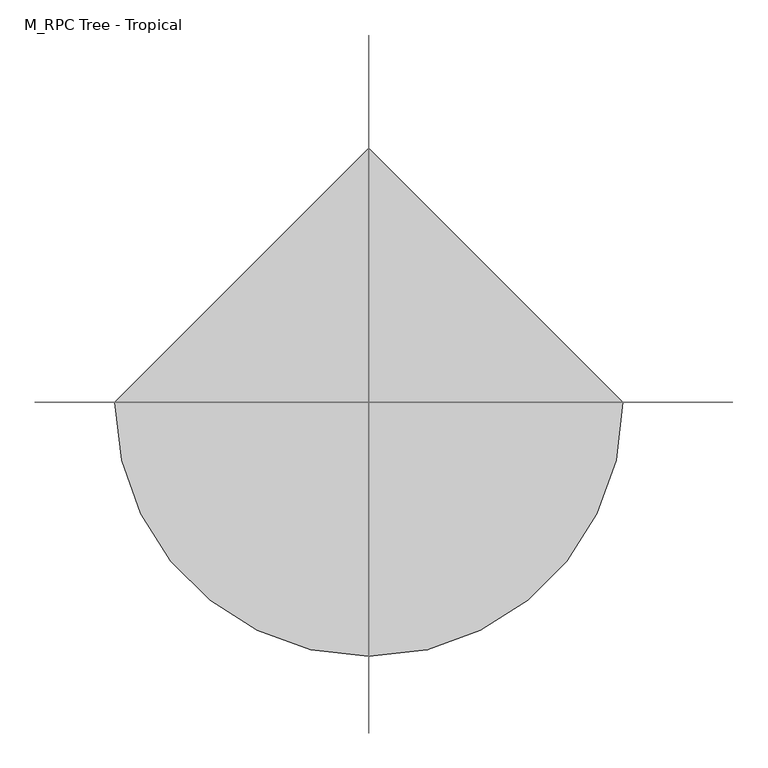
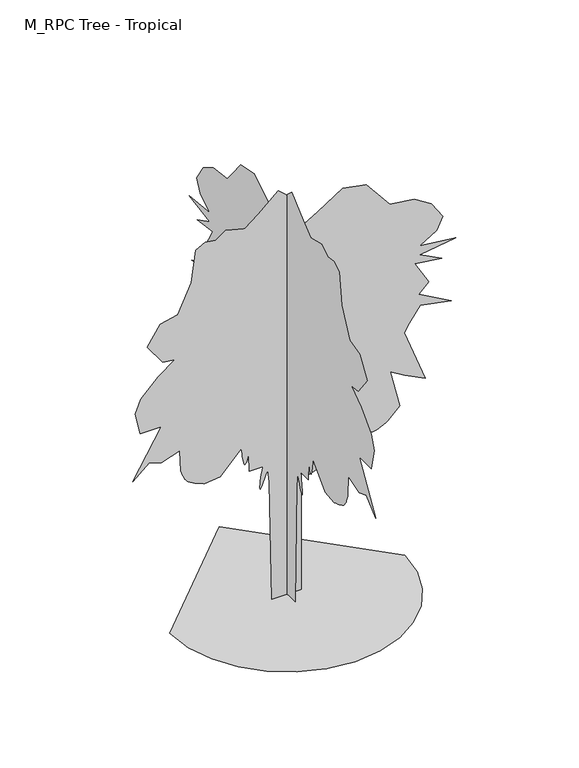
"""IFC4 building model written with IfcOpenShell, lengths in millimetres: geographic element geometry, M_RPC Tree - Tropical."""

from ifc_helpers import new_model, si_unit, origin, place, context, project, spatial, triangles, source, transform, mapped, element, save


def m_rpc_tree_tropical_0b38fe0e(model_context):
    return source(origin(), model_context, "Body", "Tessellation", [
        triangles([(-0.0239184, -79.4097514, 0.0551874), (-0.0239176, -91.9790423, 697.2397087), (-0.0239171, -101.3513263, 772.2174723), (-0.0239166, -110.6598516, 747.6798712), (-0.0239159, -119.5858783, 724.5373158), (-0.0239154, -127.7469081, 704.1797647), (-0.0239151, -134.7601792, 688.0047346), (-0.0239146, -140.2432021, 677.4021841), (-0.0239146, -143.8137145, 673.7671589), (-0.0239144, -145.0887184, 678.4947046), (-0.0239144, -144.6334592, 689.5071865), (-0.0239146, -143.35821, 703.469779), (-0.0239146, -141.3999538, 719.8923231), (-0.0239149, -138.8951921, 738.2798635), (-0.0239151, -135.9806806, 758.1449301), (-0.0239151, -132.7926757, 778.9949656), (-0.0239154, -129.4681603, 800.3350874), (-0.0239109, -204.4468958, 800.3350874), (-0.0239106, -207.5709057, 900.3053661), (-0.0239104, -211.5784191, 886.3978575), (-0.0239101, -215.5314481, 873.3927647), (-0.0239101, -219.3749454, 862.18778), (-0.0239099, -223.0547171, 853.6902609), (-0.0239096, -226.5159702, 848.8002251), (-0.0239094, -229.7037299, 848.4176903), (-0.0239091, -232.5637479, 853.4452177), (-0.0239091, -235.1505086, 862.662751), (-0.0239089, -237.5732532, 874.0103142), (-0.0239089, -239.8595235, 887.1353125), (-0.0239086, -242.0362802, 901.6828983), (-0.0239086, -244.1312831, 917.2929193), (-0.0239084, -246.1715292, 933.6154696), (-0.0239084, -248.1842879, 950.2930126), (-0.0239014, -366.9011876, 825.3276752), (-0.0238961, -454.3764441, 815.9551369), (-0.0238949, -471.7089981, 822.6501497), (-0.0238939, -488.6040788, 829.3451626), (-0.0238931, -504.6241038, 836.0401754), (-0.0238921, -519.3341798, 842.7327175), (-0.0238914, -532.296688, 849.4277304), (-0.0238906, -543.0717207, 856.1227432), (-0.0238901, -551.2217683, 862.8177561), (-0.0238899, -557.5517962, 870.2402681), (-0.0238896, -563.2268131, 878.9753454), (-0.0238891, -568.3543344, 888.8028706), (-0.0238889, -573.0468169, 899.5053423), (-0.0238886, -577.4093413, 910.8629339), (-0.0238884, -581.5518574, 922.6579262), (-0.0238881, -585.5868582, 934.6704924), (-0.0238879, -591.8368764, 1056.5108751), (-0.0238816, -694.9322187, 1022.1457489), (-0.0238776, -763.6624712, 1047.1383368), (-0.0238721, -854.2602116, 965.9130621), (-0.0238816, -694.9322187, 1234.5864155), (-0.0238746, -813.6475742, 1234.5864155), (-0.0238729, -841.7651894, 1359.5492821), (-0.0238749, -810.5226196, 1437.6520729), (-0.0238806, -713.6772955, 1537.6224243), (-0.0238861, -619.9519844, 1606.3551476), (-0.0238821, -688.6822369, 1615.7252151), (-0.0238771, -773.0350096, 1731.3180141), (-0.0238814, -701.1797298, 1843.7858585), (-0.0238871, -604.3319349, 1865.6534191), (-0.0238916, -529.3542077, 2028.1090553), (-0.0238931, -504.3616199, 2212.429636), (-0.0238961, -451.2514532, 2240.5471058), (-0.0238996, -391.8937391, 2231.1745674), (-0.0239031, -335.6585815, 2271.7872047), (-0.0239094, -229.439738, 2243.6722057), (-0.0239139, -154.4612477, 2303.0299198), (-0.0239206, -41.9933852, 2399.8776421), (-0.0239259, 45.4816443, 2321.7749966), (-0.0239259, 45.4816443, 2228.0496128), (-0.0239291, 101.7153212, 2156.1968765), (-0.0239339, 179.81833, 2199.9344685), (-0.0239421, 317.2785261, 2290.5322815), (-0.0239499, 448.4914473, 2265.5397663), (-0.0239546, 529.7166856, 2165.5694149), (-0.0239576, 579.7043684, 2103.0867462), (-0.0239659, 717.1648006, 2084.3416695), (-0.0239716, 814.0125956, 2024.9839554), (-0.0239754, 876.4927935, 1928.1362331), (-0.0239734, 842.1276672, 1859.4059807), (-0.0239676, 748.4048996, 1800.0482666), (-0.0239796, 948.3480005, 1778.180706), (-0.0239676, 748.4048996, 1746.9381363), (-0.0239749, 870.2452824, 1684.4553223), (-0.0239661, 720.2872845, 1703.200399), (-0.0239706, 798.3900753, 1568.864994), (-0.0239674, 742.1573885, 1515.7548637), (-0.0239781, 923.3554853, 1412.6595577), (-0.0239679, 751.5299269, 1447.0246113), (-0.0239641, 689.0471855, 1362.674382), (-0.0239624, 660.9296431, 1315.8116901), (-0.0239696, 779.6449986, 1006.5256994), (-0.0239626, 664.0545977, 1062.7609297), (-0.0239579, 582.8268522, 1112.7460327), (-0.0239609, 635.9370552, 894.057855), (-0.0239571, 570.33183, 828.4526299), (-0.0239564, 557.6242845, 821.1375967), (-0.0239556, 545.0017264, 814.1250887), (-0.0239549, 532.5416948, 807.7126167), (-0.0239541, 520.3266701, 802.2025606), (-0.0239534, 508.4416397, 797.8950474), (-0.0239526, 496.9641063, 795.0875153), (-0.0239521, 485.9815644, 794.0875763), (-0.0239514, 475.0865172, 794.9075117), (-0.0239509, 463.8664899, 797.2025751), (-0.0239501, 452.371443, 800.727578), (-0.0239494, 440.6588948, 805.235079), (-0.0239486, 428.7813858, 810.4825785), (-0.0239479, 416.7938181, 816.2200916), (-0.0239471, 404.7537827, 822.202648), (-0.0239471, 401.3562793, 826.1926661), (-0.0239469, 397.6587579, 830.0176506), (-0.0239466, 393.358766, 833.5151842), (-0.0239461, 388.1587564, 836.5227041), (-0.0239459, 381.7562038, 838.872706), (-0.0239454, 373.8486923, 840.4026999), (-0.0239449, 364.1411817, 840.9477247), (-0.0239441, 351.5161165, 842.4051939), (-0.0239431, 335.4485653, 846.4851774), (-0.0239419, 316.5135292, 852.7527454), (-0.0239406, 295.2834479, 860.7677359), (-0.0239394, 272.33087, 870.0952915), (-0.0239379, 248.2297975, 880.295323), (-0.0239364, 223.5557221, 890.9328278), (-0.0239341, 182.9423399, 844.0726793), (-0.0239341, 182.9423399, 765.9699612), (-0.0239354, 204.8106636, 690.9921976), (-0.0239309, 129.8324186, 665.9996098), (-0.0239281, 86.0950265, 787.8375217), (-0.0239286, 86.7090242, 0.0), (-656.1204889, -2.5e-06, 0.2095084), (-638.7804136, -150.2749844, 0.2095089), (-589.4027226, -288.2784249, 0.2095104), (-511.9349585, -410.0563296, 0.2095127), (-410.3371264, -511.6566324, 0.2095157), (-288.559258, -589.1218895, 0.2095194), (-150.5555632, -638.4995441, 0.2095234), (-0.2807655, -655.8396194, 0.2095279), (149.9941512, -638.4995441, 0.2095324), (287.9975917, -589.1218895, 0.2095364), (409.7754965, -511.6541253, 0.2095402), (511.3757993, -410.0563296, 0.2095432), (588.8410563, -288.2784249, 0.2095454), (638.2186747, -150.27473, 0.2095469), (655.55875, 5.73e-05, 0.2095474), (-0.2808805, 655.8396194, 0.2095279), (-87.7383582, 0.0001432, 0.1864386), (-100.3076491, 0.000104, 697.3697153), (-109.6799332, 9.81e-05, 772.3499496), (-118.9884584, 0.0001008, 747.8124212), (-127.9144851, 0.0001007, 724.6673223), (-136.0752606, 0.0001035, 704.3122421), (-143.0885407, 0.0001033, 688.1346685), (-148.5717998, 0.0001032, 677.5321907), (-152.142067, 0.0001058, 673.8996363), (-153.4173253, 0.0001027, 678.627182), (-152.9618298, 0.0001024, 689.6371931), (-151.6868168, 0.0001021, 703.5997856), (-149.7285606, 0.0001018, 720.0223297), (-147.2237989, 0.0001015, 738.4123409), (-144.3090422, 9.83e-05, 758.2774075), (-141.1212826, 9.79e-05, 779.1249722), (-137.7967671, 9.76e-05, 800.465094), (-212.7752755, 9.66e-05, 800.465094), (-215.8992854, 9.05e-05, 900.4379162), (-219.907035, 9.06e-05, 886.5303349), (-223.8598097, 9.35e-05, 873.5227713), (-227.7035613, 9.35e-05, 862.3202574), (-231.383333, 9.34e-05, 853.8227383), (-234.8443318, 9.32e-05, 848.9302317), (-238.0323458, 9.29e-05, 848.5476969), (-240.8921094, 9.25e-05, 853.5752243), (-243.4791245, 9.2e-05, 862.7927576), (-245.9018691, 9.15e-05, 874.1427916), (-248.187885, 9.09e-05, 887.2678625), (-250.364133, 9.03e-05, 901.8129049), (-252.4591541, 8.96e-05, 917.4254694), (-254.4991459, 8.89e-05, 933.7454762), (-256.5116502, 8.83e-05, 950.4230192), (-375.229531, 9.57e-05, 825.4601526), (-462.7047875, 9.68e-05, 816.0876143), (-480.0373415, 9.51e-05, 822.7801563), (-496.9324222, 9.62e-05, 829.4751692), (-512.9524472, 9.46e-05, 836.170182), (-527.6625232, 9.31e-05, 842.8651949), (-540.6250314, 9.46e-05, 849.5602077), (-551.4001004, 9.34e-05, 856.2527498), (-559.5501117, 9.25e-05, 862.9477627), (-565.8801395, 9.17e-05, 870.3702747), (-571.5551565, 9.1e-05, 879.1052794), (-576.6826778, 9.02e-05, 888.9328772), (-581.3751966, 9.23e-05, 899.6353489), (-585.7376847, 9.16e-05, 910.9929405), (-589.8802008, 9.09e-05, 922.7879328), (-593.9152379, 9.02e-05, 934.8029697), (-600.1652561, 8.02e-05, 1056.6433525), (-703.2606348, 8.35e-05, 1022.278299), (-771.9908146, 8.24e-05, 1047.2708868), (-862.5886276, 8.82e-05, 966.0430687), (-703.2606348, 7.15e-05, 1234.7164948), (-821.9759903, 7.23e-05, 1234.7164948), (-850.0936054, 6.32e-05, 1359.6818321), (-818.850963, 5.79e-05, 1437.784623), (-722.0056389, 5.21e-05, 1537.7549744), (-628.2804005, 4.98e-05, 1606.4850815), (-697.0105803, 4.92e-05, 1615.8576199), (-781.363353, 4.11e-05, 1731.4505642), (-709.5081459, 3.55e-05, 1843.9159378), (-612.660351, 3.2e-05, 1865.7859692), (-537.6825511, 2.24e-05, 2028.2389893), (-512.6899632, 1.34e-05, 2212.5620407), (-459.5797966, 1.15e-05, 2240.6796558), (-400.2220825, 1.14e-05, 2231.3071175), (-343.9869249, 9.4e-06, 2271.9197548), (-237.7683539, 1.11e-05, 2243.8021397), (-162.7896093, 7.5e-06, 2303.1598537), (-50.3217376, 3e-07, 2400.0077213), (37.1530375, 7.5e-06, 2321.9049305), (37.1530375, 1.32e-05, 2228.1821629), (93.3867235, 1.75e-05, 2156.3269558), (171.4897141, 1.45e-05, 2200.0645477), (308.9501827, 6.9e-06, 2290.6648315), (440.1631039, 1.07e-05, 2265.6723164), (521.3883422, 1.52e-05, 2165.6994942), (571.376025, 1.87e-05, 2103.2166801), (708.8363846, 2e-05, 2084.4742195), (805.6817087, 2.47e-05, 2025.1140347), (868.1644501, 3.03e-05, 1928.2686378), (833.7993238, 3.5e-05, 1859.5383854), (740.0764835, 3.71e-05, 1800.1808167), (940.0196571, 3.83e-05, 1778.31064), (740.0764835, 4.15e-05, 1747.070541), (861.9168663, 4.28e-05, 1684.5878723), (711.9589411, 4.32e-05, 1703.3329491), (790.0616592, 5.13e-05, 1568.9950733), (733.8289724, 5.36e-05, 1515.8874138), (915.0270693, 6.14e-05, 1412.7894917), (743.2015108, 5.94e-05, 1447.1571613), (680.7188421, 6.2e-05, 1362.8043159), (652.601227, 6.67e-05, 1315.9442402), (771.3165825, 8.36e-05, 1006.6582495), (655.7262543, 8.02e-05, 1062.8909363), (574.4985088, 7.72e-05, 1112.8760393), (627.6086391, 9.14e-05, 894.1903324), (562.0034866, 9.61e-05, 828.5826365), (549.2959411, 9.52e-05, 821.2701468), (536.673383, 9.71e-05, 814.2550953), (524.2133514, 9.62e-05, 807.8450941), (511.9983267, 9.81e-05, 802.3325672), (500.1132963, 9.72e-05, 798.025054), (488.6357265, 9.63e-05, 795.2200653), (477.6507139, 9.82e-05, 794.2175102), (466.7581738, 9.72e-05, 795.0375183), (455.5381465, 9.61e-05, 797.3325817), (444.0430996, 9.79e-05, 800.8575846), (432.3305514, 9.67e-05, 805.3675564), (420.4530424, 9.55e-05, 810.6125851), (408.4654747, 9.71e-05, 816.3500982), (396.4254393, 9.58e-05, 822.3351254), (393.0279359, 9.54e-05, 826.3251434), (389.3304145, 9.5e-05, 830.150128), (385.0304226, 9.45e-05, 833.6476616), (379.830413, 9.39e-05, 836.6527107), (373.4278605, 9.33e-05, 839.0027126), (365.5203489, 9.54e-05, 840.5327065), (355.8128019, 9.45e-05, 841.0802021), (343.1877731, 9.34e-05, 842.5376713), (327.1202219, 9.47e-05, 846.6177275), (308.1851495, 9.28e-05, 852.882752), (286.9550863, 9.35e-05, 860.8977425), (264.0025084, 9.41e-05, 870.2252981), (239.9011816, 9.16e-05, 880.4278004), (215.2271062, 9.2e-05, 891.0653778), (174.613724, 9.55e-05, 844.2026859), (174.613724, 9.78e-05, 766.0999678), (196.4822838, 0.000102, 691.1222042), (121.504057, 0.0001047, 666.1296164), (77.7664196, 9.71e-05, 787.9699991), (78.3804265, 0.0001436, 0.1312562)], [[85, 84, 86], [53, 52, 54], [91, 90, 92], [87, 86, 88], [95, 94, 96], [96, 94, 97], [9, 8, 10], [52, 51, 54], [51, 50, 54], [1, 133, 2], [133, 132, 2], [2, 132, 3], [131, 130, 132], [130, 129, 132], [129, 128, 132], [18, 17, 19], [71, 70, 72], [72, 70, 73], [10, 8, 11], [8, 7, 11], [11, 7, 12], [7, 6, 12], [12, 6, 13], [6, 5, 13], [13, 5, 14], [5, 4, 14], [14, 4, 15], [4, 3, 15], [15, 3, 16], [16, 3, 17], [55, 54, 56], [89, 88, 90], [56, 54, 57], [57, 54, 58], [61, 60, 62], [62, 60, 63], [60, 59, 63], [25, 24, 26], [24, 23, 26], [26, 23, 27], [23, 22, 27], [27, 22, 28], [22, 21, 28], [28, 21, 29], [21, 20, 29], [29, 20, 30], [20, 19, 30], [30, 19, 31], [82, 81, 83], [83, 81, 84], [81, 80, 84], [80, 79, 84], [70, 69, 73], [98, 97, 99], [31, 19, 32], [99, 97, 100], [58, 54, 59], [100, 97, 101], [101, 97, 102], [102, 97, 103], [103, 97, 104], [104, 97, 105], [105, 97, 106], [106, 97, 107], [107, 97, 108], [108, 97, 109], [109, 97, 110], [110, 97, 111], [111, 97, 112], [112, 97, 113], [113, 97, 114], [114, 97, 115], [115, 97, 116], [116, 97, 117], [117, 97, 118], [118, 97, 119], [119, 97, 120], [120, 97, 121], [121, 97, 122], [122, 97, 123], [123, 97, 124], [124, 97, 125], [125, 97, 126], [126, 97, 127], [65, 64, 66], [66, 64, 67], [68, 67, 69], [67, 64, 69], [3, 132, 17], [73, 69, 74], [69, 64, 74], [64, 63, 74], [63, 59, 74], [17, 132, 19], [132, 128, 19], [128, 127, 19], [92, 90, 93], [76, 75, 77], [77, 75, 78], [78, 75, 79], [79, 75, 84], [75, 74, 84], [74, 59, 84], [84, 59, 86], [86, 59, 88], [88, 59, 90], [90, 59, 93], [93, 59, 94], [94, 59, 97], [97, 59, 127], [127, 59, 19], [32, 19, 33], [19, 59, 33], [59, 54, 33], [54, 50, 33], [33, 50, 34], [50, 49, 34], [34, 49, 35], [35, 49, 36], [36, 49, 37], [49, 48, 37], [37, 48, 38], [48, 47, 38], [38, 47, 39], [47, 46, 39], [39, 46, 40], [46, 45, 40], [45, 44, 40], [40, 44, 41], [44, 43, 41], [41, 43, 42], [148, 149, 134], [147, 148, 134], [147, 134, 135], [146, 147, 135], [146, 135, 136], [146, 136, 137], [145, 146, 137], [144, 145, 137], [144, 137, 138], [144, 138, 139], [144, 139, 140], [144, 140, 141], [144, 141, 142], [144, 142, 143], [233, 234, 235], [201, 202, 203], [239, 240, 241], [235, 236, 237], [243, 244, 245], [243, 245, 246], [157, 158, 159], [200, 201, 203], [199, 200, 203], [282, 150, 151], [281, 282, 151], [281, 151, 152], [279, 280, 281], [278, 279, 281], [277, 278, 281], [166, 167, 168], [219, 220, 221], [219, 221, 222], [157, 159, 160], [156, 157, 160], [156, 160, 161], [155, 156, 161], [155, 161, 162], [154, 155, 162], [154, 162, 163], [153, 154, 163], [153, 163, 164], [152, 153, 164], [152, 164, 165], [152, 165, 166], [203, 204, 205], [237, 238, 239], [203, 205, 206], [203, 206, 207], [209, 210, 211], [209, 211, 212], [208, 209, 212], [173, 174, 175], [172, 173, 175], [172, 175, 176], [171, 172, 176], [171, 176, 177], [170, 171, 177], [170, 177, 178], [169, 170, 178], [169, 178, 179], [168, 169, 179], [168, 179, 180], [230, 231, 232], [230, 232, 233], [229, 230, 233], [228, 229, 233], [218, 219, 222], [246, 247, 248], [168, 180, 181], [246, 248, 249], [203, 207, 208], [246, 249, 250], [246, 250, 251], [246, 251, 252], [246, 252, 253], [246, 253, 254], [246, 254, 255], [246, 255, 256], [246, 256, 257], [246, 257, 258], [246, 258, 259], [246, 259, 260], [246, 260, 261], [246, 261, 262], [246, 262, 263], [246, 263, 264], [246, 264, 265], [246, 265, 266], [246, 266, 267], [246, 267, 268], [246, 268, 269], [246, 269, 270], [246, 270, 271], [246, 271, 272], [246, 272, 273], [246, 273, 274], [246, 274, 275], [246, 275, 276], [213, 214, 215], [213, 215, 216], [216, 217, 218], [213, 216, 218], [281, 152, 166], [218, 222, 223], [213, 218, 223], [212, 213, 223], [208, 212, 223], [281, 166, 168], [277, 281, 168], [276, 277, 168], [239, 241, 242], [224, 225, 226], [224, 226, 227], [224, 227, 228], [224, 228, 233], [223, 224, 233], [208, 223, 233], [208, 233, 235], [208, 235, 237], [208, 237, 239], [208, 239, 242], [208, 242, 243], [208, 243, 246], [208, 246, 276], [208, 276, 168], [168, 181, 182], [208, 168, 182], [203, 208, 182], [199, 203, 182], [199, 182, 183], [198, 199, 183], [198, 183, 184], [198, 184, 185], [198, 185, 186], [197, 198, 186], [197, 186, 187], [196, 197, 187], [196, 187, 188], [195, 196, 188], [195, 188, 189], [194, 195, 189], [193, 194, 189], [193, 189, 190], [192, 193, 190], [192, 190, 191]], closed=False),
    ])


if __name__ == "__main__":
    model = new_model("IFC4")
    model_context = context("Model", 3, world=origin())
    ifc_project = project(units=[si_unit("LENGTHUNIT", "METRE", prefix="MILLI")], contexts=[model_context])
    site = spatial("IfcSite", under=ifc_project)
    building = spatial("IfcBuilding", under=site)
    placement = place(None, origin())
    m_rpc_tree_tropical_shape = m_rpc_tree_tropical_0b38fe0e(model_context)
    element("IfcGeographicElement", 1, ObjectType="M_RPC Tree - Tropical", at=placement, inside=building, context=model_context, shape_type="MappedRepresentation", body=[
        mapped(m_rpc_tree_tropical_shape, transform((0.0, 0.0, 0.0), x_axis=(1.0, 0.0, 0.0), y_axis=(0.0, 1.0, 0.0), z_axis=(0.0, 0.0, 1.0))),
    ])
    save(model, "model.ifc")

# Revit data of these elements
# Type "M_RPC Tree - Tropical"
#   built-in parameter 1005198 = "{2, 15},{39, RPC-16-G2MF-J1Q0-CAN1-N000-ST1L-LVER-AU},{1, 0},{1, 0},{2, 35},{1, 8},{5, Color},{1, 0},{1, 0},{3, 0.8},{3, 0.8},{3, 0.8},{1, 8},{7, BBoxMin},{1, 0},{1, 0},{1, 0},{1, 0},{1, 0},{1, 8},{7, BBoxMax},{1, 0},{1, 0},{1, 0},{1, 0},{1, 0},{2, 11},{9, RPCTypeId},{1, 0},{1, 0},{39, RPC-16-G2MF-J1Q0-CAN1-N000-ST1L-LVER-AU},{1, 6},{14, RPCPlantHeight},{1, 0},{1, 0},{7, 7.87402},{2, 11},{7, keyword},{1, 0},{1, 0},{75, :Geometry:RPC:Windmill Palm:Trachycarpus fortunei:in habitat:palm:tropical.},{2, 11},{8, category},{1, 0},{1, 0},{17, :Trees [Tropical]},{2, 11},{12, LocalizedUID},{1, 0},{1, 0},{13, Windmill Palm},{2, 14},{6, Height},{1, 0},{1, 0},{7, 7.87402},{1, 2},{16, Cast Reflections},{1, 0},{1, 0},{1, 0},{1, 2},{12, Cast Shadows},{1, 0},{1, 0},{1, 1},{1, 2},{9, Lock View},{1, 0},{1, 0},{1, 0},{1, 4},{5, ViewC},{1, 0},{1, 0},{1, 0},{2, 11},{20, AdvancedUIDefinition},{1, 0},{1, 0},{0, },{2, 11},{10, AssetLibID},{1, 0},{1, 0},{36, 4D3F6E72-3F99-4203-98E9-AF80B3C7A7A4},{2, 11},{10, BaseSchema},{1, 0},{1, 0},{9, RPCSchema},{2, 11},{12, ExchangeGUID},{1, 0},{1, 0},{0, },{1, 2},{6, Hidden},{1, 0},{1, 0},{1, 0},{1, 4},{11, RPCCategory},{1, 0},{1, 0},{1, 0},{2, 11},{8, RPCImage},{1, 0},{1, 0},{0, },{1, 4},{13, SchemaVersion},{1, 0},{1, 0},{1, 4},{2, 11},{12, UIDefinition},{1, 0},{1, 0},{0, },{2, 11},{6, UIName},{1, 0},{1, 0},{39, RPC-16-G2MF-J1Q0-CAN1-N000-ST1L-LVER-AU},{2, 11},{11, VersionGUID},{1, 0},{1, 0},{9, RPCSchema},{2, 11},{9, assettype},{1, 0},{1, 0},{11, RPCGeometry},{2, 11},{11, description},{1, 0},{1, 0},{0, },{2, 11},{9, localname},{1, 0},{1, 0},{3, RPC},{2, 11},{9, localtype},{1, 0},{1, 0},{3, RPC},{1, 4},{8, revision},{1, 0},{1, 0},{1, 1},{2, 11},{9, thumbnail},{1, 0},{1, 0},{0, },{1, 4},{7, version},{1, 0},{1, 0},{1, 1},{1, 2},{20, RPC_Cast Reflections},{1, 0},{1, 0},{1, 1},{1, 2},{16, RPC_Cast Shadows},{1, 0},{1, 0},{1, 1},{1, 2},{13, RPC_Lock View},{1, 0},{1, 0},{1, 0},{1, 4},{9, RPC_ViewC},{1, 0},{1, 0},{1, 0},{21, assetlibrary_base.fbx},{1, 5},"
#   built-in parameter 1005195 = "RPC-16-G2MF-J1Q0-CAN1-N000-ST1L-LVER-AU"
#   Height = 2400 mm
#   Plan Symbol = element 405753
#   Description = (empty or 0)
#   Default Elevation = 0
